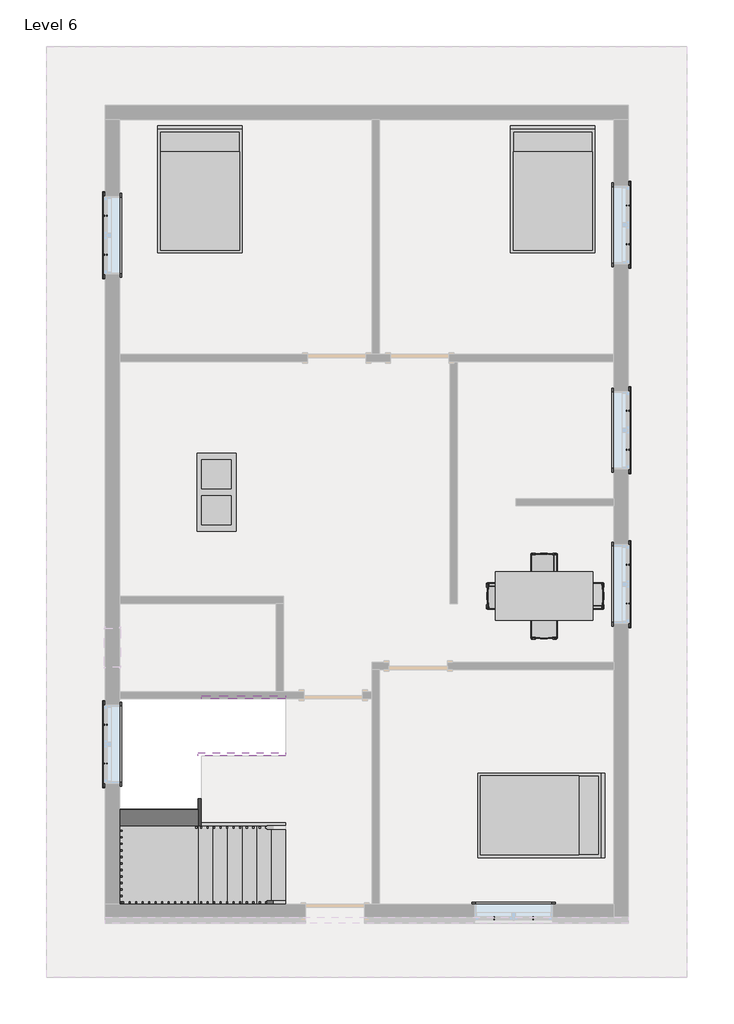
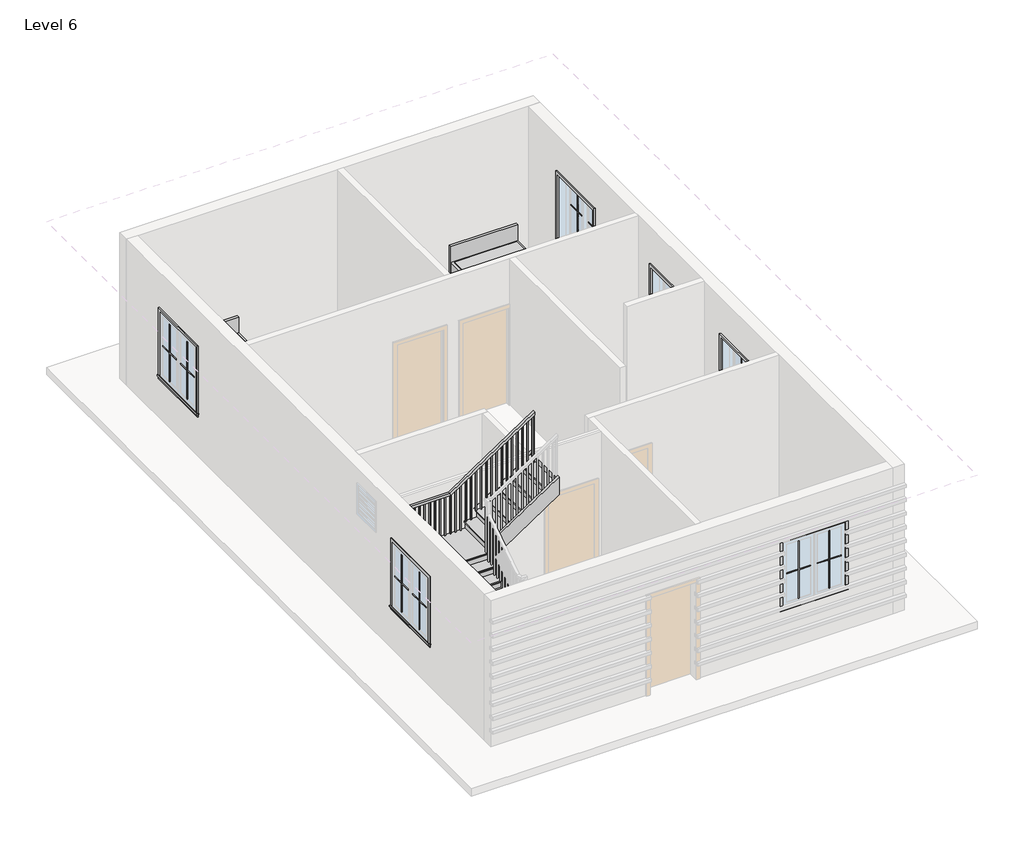
# One storey, part 3 of 3: 25 proxies, 5 members, 4 furniture elements, 1 railing, 1 stair flight.
"""IFC4 building model written with IfcOpenShell, lengths in millimetres."""

from ifc_helpers import new_model, si_unit, frame, origin, place, context, project, spatial, polyline, outline, extrude, faceted_brep, transform, mapped, element, save
from components import muntin_pattern_2x2_muntin_pattern_2x2_ba8901dc, muntin_pattern_2x2_muntin_pattern_2x2_877df4e9, trim_window_exterior_flat_with_sill_fda35bc9, trim_window_interior_flat_picture_frame_a80dbcd9, coffee_table_with_brass_mullions_11320_coffee_table_with_5962bef7, bed_17739_bed_17739_15c61121, dining_table_w_chairs_11374_0cdfc61b, stair_flight_f9fade56

model = new_model("IFC4")

# Units and contexts
model_context = context("Model", 3, world=origin())
ifc_project = project(units=[si_unit("LENGTHUNIT", "METRE", prefix="MILLI")], contexts=[model_context])

# Site, building, storey
site = spatial("IfcSite", under=ifc_project)
building = spatial("IfcBuilding", under=site)
storey = spatial("IfcBuildingStorey", under=building, Name="Level 6", Elevation=15849.6)

# Proxies
placement = place(None, origin())
muntin_pattern_2x2_muntin_pattern_2x2_shape = muntin_pattern_2x2_muntin_pattern_2x2_ba8901dc(model_context)
element("IfcBuildingElementProxy", 1, Name="Muntin Pattern_2x2 : Muntin Pattern_2x2", ObjectType="Muntin Pattern_2x2 : Muntin Pattern_2x2", at=placement, inside=storey, context=model_context, shape_type="MappedRepresentation", body=[
    mapped(muntin_pattern_2x2_muntin_pattern_2x2_shape, transform((-5325.0867403, -4189.9051559, 16833.85), x_axis=(0.0, 1.0, 0.0), y_axis=(-1.0, 0.0, 0.0), z_axis=(0.0, 0.0, 1.0))),
])
element("IfcBuildingElementProxy", 2, Name="Muntin Pattern_2x2 : Muntin Pattern_2x2", ObjectType="Muntin Pattern_2x2 : Muntin Pattern_2x2", at=placement, inside=storey, context=model_context, shape_type="MappedRepresentation", body=[
    mapped(muntin_pattern_2x2_muntin_pattern_2x2_shape, transform((-5325.0867403, 3744.4198441, 16833.85), x_axis=(0.0, 1.0, 0.0), y_axis=(-1.0, 0.0, 0.0), z_axis=(0.0, 0.0, 1.0))),
])
element("IfcBuildingElementProxy", 3, Name="Muntin Pattern_2x2 : Muntin Pattern_2x2", ObjectType="Muntin Pattern_2x2 : Muntin Pattern_2x2", at=placement, inside=storey, context=model_context, shape_type="MappedRepresentation", body=[
    mapped(muntin_pattern_2x2_muntin_pattern_2x2_shape, transform((2821.9632597, 4512.7698441, 16833.85), x_axis=(0.0, -1.0, 0.0), y_axis=(1.0, 0.0, 0.0), z_axis=(0.0, 0.0, 1.0))),
])
element("IfcBuildingElementProxy", 4, Name="Muntin Pattern_2x2 : Muntin Pattern_2x2", ObjectType="Muntin Pattern_2x2 : Muntin Pattern_2x2", at=placement, inside=storey, context=model_context, shape_type="MappedRepresentation", body=[
    mapped(muntin_pattern_2x2_muntin_pattern_2x2_shape, transform((2821.9632597, 1312.3698441, 16833.85), x_axis=(0.0, -1.0, 0.0), y_axis=(1.0, 0.0, 0.0), z_axis=(0.0, 0.0, 1.0))),
])
element("IfcBuildingElementProxy", 5, Name="Muntin Pattern_2x2 : Muntin Pattern_2x2", ObjectType="Muntin Pattern_2x2 : Muntin Pattern_2x2", at=placement, inside=storey, context=model_context, shape_type="MappedRepresentation", body=[
    mapped(muntin_pattern_2x2_muntin_pattern_2x2_shape, transform((2821.9632597, -1087.9301559, 16833.85), x_axis=(0.0, -1.0, 0.0), y_axis=(1.0, 0.0, 0.0), z_axis=(0.0, 0.0, 1.0))),
])
element("IfcBuildingElementProxy", 6, Name="Muntin Pattern_2x2 : Muntin Pattern_2x2", ObjectType="Muntin Pattern_2x2 : Muntin Pattern_2x2", at=placement, inside=storey, context=model_context, shape_type="MappedRepresentation", body=[
    mapped(muntin_pattern_2x2_muntin_pattern_2x2_shape, transform((1344.0007597, -6601.3176559, 16833.85), x_axis=(-1.0, 0.0, 0.0), y_axis=(0.0, -1.0, 0.0), z_axis=(0.0, 0.0, 1.0))),
])
muntin_pattern_2x2_muntin_pattern_2x2_2_shape = muntin_pattern_2x2_muntin_pattern_2x2_877df4e9(model_context)
element("IfcBuildingElementProxy", 7, Name="Muntin Pattern_2x2 : Muntin Pattern_2x2", ObjectType="Muntin Pattern_2x2 : Muntin Pattern_2x2", at=placement, inside=storey, context=model_context, shape_type="MappedRepresentation", body=[
    mapped(muntin_pattern_2x2_muntin_pattern_2x2_2_shape, transform((-5325.0867403, -3583.4801559, 16833.85), x_axis=(0.0, -1.0, 0.0), y_axis=(1.0, 0.0, 0.0), z_axis=(0.0, 0.0, 1.0))),
])
element("IfcBuildingElementProxy", 8, Name="Muntin Pattern_2x2 : Muntin Pattern_2x2", ObjectType="Muntin Pattern_2x2 : Muntin Pattern_2x2", at=placement, inside=storey, context=model_context, shape_type="MappedRepresentation", body=[
    mapped(muntin_pattern_2x2_muntin_pattern_2x2_2_shape, transform((-5325.0867403, 4350.8448441, 16833.85), x_axis=(0.0, -1.0, 0.0), y_axis=(1.0, 0.0, 0.0), z_axis=(0.0, 0.0, 1.0))),
])
element("IfcBuildingElementProxy", 9, Name="Muntin Pattern_2x2 : Muntin Pattern_2x2", ObjectType="Muntin Pattern_2x2 : Muntin Pattern_2x2", at=placement, inside=storey, context=model_context, shape_type="MappedRepresentation", body=[
    mapped(muntin_pattern_2x2_muntin_pattern_2x2_2_shape, transform((2821.9632597, 3906.3448441, 16833.85), x_axis=(0.0, 1.0, 0.0), y_axis=(-1.0, 0.0, 0.0), z_axis=(0.0, 0.0, 1.0))),
])
element("IfcBuildingElementProxy", 10, Name="Muntin Pattern_2x2 : Muntin Pattern_2x2", ObjectType="Muntin Pattern_2x2 : Muntin Pattern_2x2", at=placement, inside=storey, context=model_context, shape_type="MappedRepresentation", body=[
    mapped(muntin_pattern_2x2_muntin_pattern_2x2_2_shape, transform((2821.9632597, 705.9448441, 16833.85), x_axis=(0.0, 1.0, 0.0), y_axis=(-1.0, 0.0, 0.0), z_axis=(0.0, 0.0, 1.0))),
])
element("IfcBuildingElementProxy", 11, Name="Muntin Pattern_2x2 : Muntin Pattern_2x2", ObjectType="Muntin Pattern_2x2 : Muntin Pattern_2x2", at=placement, inside=storey, context=model_context, shape_type="MappedRepresentation", body=[
    mapped(muntin_pattern_2x2_muntin_pattern_2x2_2_shape, transform((2821.9632597, -1694.3551559, 16833.85), x_axis=(0.0, 1.0, 0.0), y_axis=(-1.0, 0.0, 0.0), z_axis=(0.0, 0.0, 1.0))),
])
element("IfcBuildingElementProxy", 12, Name="Muntin Pattern_2x2 : Muntin Pattern_2x2", ObjectType="Muntin Pattern_2x2 : Muntin Pattern_2x2", at=placement, inside=storey, context=model_context, shape_type="MappedRepresentation", body=[
    mapped(muntin_pattern_2x2_muntin_pattern_2x2_2_shape, transform((737.5757597, -6601.3176559, 16833.85), x_axis=(1.0, 0.0, 0.0), y_axis=(0.0, 1.0, 0.0), z_axis=(0.0, 0.0, 1.0))),
])
trim_window_exterior_flat_with_sill_shape = trim_window_exterior_flat_with_sill_fda35bc9(model_context)
element("IfcBuildingElementProxy", 13, Name="Trim-Window-Exterior-Flat : with Sill", ObjectType="Trim-Window-Exterior-Flat : with Sill", at=placement, inside=storey, context=model_context, shape_type="MappedRepresentation", body=[
    mapped(trim_window_exterior_flat_with_sill_shape, transform((-5334.6117403, -3886.6926559, 18110.2), x_axis=(0.0, -1.0, 0.0), y_axis=(0.0, 0.0, 1.0), z_axis=(-1.0, 0.0, 0.0))),
])
element("IfcBuildingElementProxy", 14, Name="Trim-Window-Exterior-Flat : with Sill", ObjectType="Trim-Window-Exterior-Flat : with Sill", at=placement, inside=storey, context=model_context, shape_type="MappedRepresentation", body=[
    mapped(trim_window_exterior_flat_with_sill_shape, transform((-5334.6117403, 4047.6323441, 18110.2), x_axis=(0.0, -1.0, 0.0), y_axis=(0.0, 0.0, 1.0), z_axis=(-1.0, 0.0, 0.0))),
])
element("IfcBuildingElementProxy", 15, Name="Trim-Window-Exterior-Flat : with Sill", ObjectType="Trim-Window-Exterior-Flat : with Sill", at=placement, inside=storey, context=model_context, shape_type="MappedRepresentation", body=[
    mapped(trim_window_exterior_flat_with_sill_shape, transform((2831.4882597, 4209.5573441, 18110.2), x_axis=(0.0, 1.0, 0.0), y_axis=(0.0, 0.0, 1.0), z_axis=(1.0, 0.0, 0.0))),
])
element("IfcBuildingElementProxy", 16, Name="Trim-Window-Exterior-Flat : with Sill", ObjectType="Trim-Window-Exterior-Flat : with Sill", at=placement, inside=storey, context=model_context, shape_type="MappedRepresentation", body=[
    mapped(trim_window_exterior_flat_with_sill_shape, transform((2831.4882597, 1009.1573441, 18110.2), x_axis=(0.0, 1.0, 0.0), y_axis=(0.0, 0.0, 1.0), z_axis=(1.0, 0.0, 0.0))),
])
element("IfcBuildingElementProxy", 17, Name="Trim-Window-Exterior-Flat : with Sill", ObjectType="Trim-Window-Exterior-Flat : with Sill", at=placement, inside=storey, context=model_context, shape_type="MappedRepresentation", body=[
    mapped(trim_window_exterior_flat_with_sill_shape, transform((2831.4882597, -1391.1426559, 18110.2), x_axis=(0.0, 1.0, 0.0), y_axis=(0.0, 0.0, 1.0), z_axis=(1.0, 0.0, 0.0))),
])
element("IfcBuildingElementProxy", 18, Name="Trim-Window-Exterior-Flat : with Sill", ObjectType="Trim-Window-Exterior-Flat : with Sill", at=placement, inside=storey, context=model_context, shape_type="MappedRepresentation", body=[
    mapped(trim_window_exterior_flat_with_sill_shape, transform((1040.7882597, -6610.8426559, 18110.2), x_axis=(1.0, 0.0, 0.0), y_axis=(0.0, 0.0, 1.0), z_axis=(0.0, -1.0, 0.0))),
])
trim_window_interior_flat_picture_frame_shape = trim_window_interior_flat_picture_frame_a80dbcd9(model_context)
element("IfcBuildingElementProxy", 19, Name="Trim-Window-Interior-Flat : Picture Frame", ObjectType="Trim-Window-Interior-Flat : Picture Frame", at=placement, inside=storey, context=model_context, shape_type="MappedRepresentation", body=[
    mapped(trim_window_interior_flat_picture_frame_shape, transform((-5106.0117403, -3886.6926559, 18110.2), x_axis=(0.0, 1.0, 0.0), y_axis=(0.0, 0.0, 1.0), z_axis=(1.0, 0.0, 0.0))),
])
element("IfcBuildingElementProxy", 20, Name="Trim-Window-Interior-Flat : Picture Frame", ObjectType="Trim-Window-Interior-Flat : Picture Frame", at=placement, inside=storey, context=model_context, shape_type="MappedRepresentation", body=[
    mapped(trim_window_interior_flat_picture_frame_shape, transform((-5106.0117403, 4047.6323441, 18110.2), x_axis=(0.0, 1.0, 0.0), y_axis=(0.0, 0.0, 1.0), z_axis=(1.0, 0.0, 0.0))),
])
element("IfcBuildingElementProxy", 21, Name="Trim-Window-Interior-Flat : Picture Frame", ObjectType="Trim-Window-Interior-Flat : Picture Frame", at=placement, inside=storey, context=model_context, shape_type="MappedRepresentation", body=[
    mapped(trim_window_interior_flat_picture_frame_shape, transform((2602.8882597, 4209.5573441, 18110.2), x_axis=(0.0, -1.0, 0.0), y_axis=(0.0, 0.0, 1.0), z_axis=(-1.0, 0.0, 0.0))),
])
element("IfcBuildingElementProxy", 22, Name="Trim-Window-Interior-Flat : Picture Frame", ObjectType="Trim-Window-Interior-Flat : Picture Frame", at=placement, inside=storey, context=model_context, shape_type="MappedRepresentation", body=[
    mapped(trim_window_interior_flat_picture_frame_shape, transform((2602.8882597, 1009.1573441, 18110.2), x_axis=(0.0, -1.0, 0.0), y_axis=(0.0, 0.0, 1.0), z_axis=(-1.0, 0.0, 0.0))),
])
element("IfcBuildingElementProxy", 23, Name="Trim-Window-Interior-Flat : Picture Frame", ObjectType="Trim-Window-Interior-Flat : Picture Frame", at=placement, inside=storey, context=model_context, shape_type="MappedRepresentation", body=[
    mapped(trim_window_interior_flat_picture_frame_shape, transform((2602.8882597, -1391.1426559, 18110.2), x_axis=(0.0, -1.0, 0.0), y_axis=(0.0, 0.0, 1.0), z_axis=(-1.0, 0.0, 0.0))),
])
element("IfcBuildingElementProxy", 24, Name="Trim-Window-Interior-Flat : Picture Frame", ObjectType="Trim-Window-Interior-Flat : Picture Frame", at=placement, inside=storey, context=model_context, shape_type="MappedRepresentation", body=[
    mapped(trim_window_interior_flat_picture_frame_shape, transform((1040.7882597, -6382.2426559, 18110.2), x_axis=(-1.0, 0.0, 0.0), y_axis=(0.0, 0.0, 1.0), z_axis=(0.0, 1.0, 0.0))),
])
coffee_table_with_brass_mullions_11320_coffee_table_with_shape = coffee_table_with_brass_mullions_11320_coffee_table_with_5962bef7(model_context)
element("IfcBuildingElementProxy", 25, Name="coffee_table_with_brass_mullions_11320 : coffee_table_with_brass_mullions_11320", ObjectType="coffee_table_with_brass_mullions_11320 : coffee_table_with_brass_mullions_11320", at=placement, inside=storey, context=model_context, shape_type="MappedRepresentation", body=[
    mapped(coffee_table_with_brass_mullions_11320_coffee_table_with_shape, transform((-3162.9117403, 678.9573441, 15849.6), x_axis=(0.0, 1.0, 0.0), y_axis=(-1.0, 0.0, 0.0), z_axis=(0.0, 0.0, 1.0))),
])

# Furniture
bed_17739_bed_17739_shape = bed_17739_bed_17739_15c61121(model_context)
element("IfcFurniture", 26, ObjectType="Bed_17739 : Bed_17739", at=placement, inside=storey, context=model_context, shape_type="MappedRepresentation", body=[
    mapped(bed_17739_bed_17739_shape, transform((-3855.0617403, 4742.9573441, 15849.6), x_axis=(1.0, 0.0, 0.0), y_axis=(0.0, 1.0, 0.0), z_axis=(0.0, 0.0, 1.0))),
])
element("IfcFurniture", 27, ObjectType="Bed_17739 : Bed_17739", at=placement, inside=storey, context=model_context, shape_type="MappedRepresentation", body=[
    mapped(bed_17739_bed_17739_shape, transform((1650.3882597, 4742.9573441, 15849.6), x_axis=(1.0, 0.0, 0.0), y_axis=(0.0, 1.0, 0.0), z_axis=(0.0, 0.0, 1.0))),
])
element("IfcFurniture", 28, ObjectType="Bed_17739 : Bed_17739", at=placement, inside=storey, context=model_context, shape_type="MappedRepresentation", body=[
    mapped(bed_17739_bed_17739_shape, transform((1447.1882597, -4997.9426559, 15849.6), x_axis=(0.0, -1.0, 0.0), y_axis=(1.0, 0.0, 0.0), z_axis=(0.0, 0.0, 1.0))),
])
dining_table_w_chairs_11374_shape = dining_table_w_chairs_11374_0cdfc61b(model_context)
element("IfcFurniture", 29, ObjectType="Dining_Table_w_Chairs_11374", at=placement, inside=storey, context=model_context, shape_type="MappedRepresentation", body=[
    mapped(dining_table_w_chairs_11374_shape, transform((1497.0410232, -1671.6886654, 15849.6), x_axis=(1.0, 0.0, 0.0), y_axis=(0.0, 1.0, 0.0), z_axis=(0.0, 0.0, 1.0))),
])

# Members
element("IfcMember", 30, ObjectType="Stringer - 2\" Width", at=placement, inside=storey, context=model_context, shape_type="SweptSolid", body=[
    extrude(outline(polyline([(15849.6, -2515.2117403), (16067.6398409, -2515.2117403), (16321.6398409, -2896.2117403), (16321.6398409, -3445.6977546), (15849.6, -2737.6379933), (15849.6, -2515.2117403)])), frame((0.0, -6433.0426559, 0.0), z_axis=(0.0, 1.0, 0.0), x_axis=(0.0, 0.0, 1.0)), (0.0, 0.0, 1.0), 50.8),
])
element("IfcMember", 31, ObjectType="Stringer - 2\" Width", at=placement, inside=storey, context=model_context, shape_type="SweptSolid", body=[
    extrude(outline(polyline([(18088.9158313, -3277.2117403), (18596.9158313, -2515.2117403), (18963.2398409, -2515.2117403), (18088.9158313, -3826.6977546), (18088.9158313, -3277.2117403)])), frame((0.0, -3181.8426559, 0.0), z_axis=(0.0, 1.0, 0.0), x_axis=(0.0, 0.0, 1.0)), (0.0, 0.0, 1.0), 50.8),
])
element("IfcMember", 32, ObjectType="Stringer - 2\" Width", at=placement, inside=storey, context=model_context, shape_type="SweptSolid", body=[
    extrude(outline(polyline([(15849.6, -2515.2117403), (16067.6398409, -2515.2117403), (16948.1731743, -3836.0117403), (16581.8491647, -3836.0117403), (15849.6, -2737.6379933), (15849.6, -2515.2117403)])), frame((0.0, -5163.0426559, 0.0), z_axis=(0.0, 1.0, 0.0), x_axis=(0.0, 0.0, 1.0)), (0.0, 0.0, 1.0), 50.8),
])
element("IfcMember", 33, ObjectType="Stringer - 2\" Width", at=placement, inside=storey, context=model_context, shape_type="SweptSolid", body=[
    extrude(outline(polyline([(-5163.0426559, 16768.1158313), (-5163.0426559, 17134.4398409), (-4070.8426559, 17862.5731743), (-4070.8426559, 17496.2491647), (-5163.0426559, 16768.1158313)])), frame((-3886.8117403, 0.0, 0.0), z_axis=(1.0, 0.0, 0.0), x_axis=(0.0, 1.0, 0.0)), (0.0, 0.0, 1.0), 50.8),
])
element("IfcMember", 34, ObjectType="Stringer - 2\" Width", at=placement, inside=storey, context=model_context, shape_type="SweptSolid", body=[
    extrude(outline(polyline([(18048.8398409, -3886.8117403), (17682.5158313, -3886.8117403), (18596.9158313, -2515.2117403), (18963.2398409, -2515.2117403), (18048.8398409, -3886.8117403)])), frame((0.0, -4070.8426559, 0.0), z_axis=(0.0, 1.0, 0.0), x_axis=(0.0, 0.0, 1.0)), (0.0, 0.0, 1.0), 50.8),
])

# Railing
element("IfcRailing", 35, ObjectType="Handrail - Rectangular", at=placement, inside=storey, context=model_context, shape_type="SolidModel", body=[
    faceted_brep([(-2515.2117403, -6382.2426559, 16916.4), (-2515.2117403, -6382.2426559, 16855.3459984), (-2515.2117403, -6331.4426559, 16855.3459984), (-2515.2117403, -6331.4426559, 16916.4), (-4001.1117403, -6382.2426559, 17907.0), (-4016.4927427, -6382.2426559, 17856.2), (-4016.4927427, -6331.4426559, 17856.2), (-4001.1117403, -6331.4426559, 17907.0), (-5106.0117403, -6382.2426559, 17907.0), (-5106.0117403, -6382.2426559, 17856.2), (-5055.2117403, -6331.4426559, 17856.2), (-5055.2117403, -6331.4426559, 17907.0), (-5106.0117403, -5277.3426559, 17907.0), (-5106.0117403, -5261.9616535, 17856.2), (-5055.2117403, -5261.9616535, 17856.2), (-5055.2117403, -5277.3426559, 17907.0), (-5106.0117403, -4096.2426559, 18694.4), (-5106.0117403, -4080.8616535, 18643.6), (-5055.2117403, -4080.8616535, 18643.6), (-5055.2117403, -4096.2426559, 18694.4), (-5106.0117403, -3181.8426559, 18694.4), (-5106.0117403, -3181.8426559, 18643.6), (-5055.2117403, -3232.6426559, 18643.6), (-5055.2117403, -3232.6426559, 18694.4), (-4191.6117403, -3181.8426559, 18694.4), (-4176.2307379, -3181.8426559, 18643.6), (-4176.2307379, -3232.6426559, 18643.6), (-4191.6117403, -3232.6426559, 18694.4), (-2515.2117403, -3181.8426559, 19812.0), (-2515.2117403, -3232.6426559, 19812.0), (-2515.2117403, -3232.6426559, 19750.9459984), (-2515.2117403, -3181.8426559, 19750.9459984)], [[[0, 1, 2, 3]], [[1, 0, 4, 5]], [[2, 1, 5, 6]], [[3, 2, 6, 7]], [[0, 3, 7, 4]], [[5, 4, 8, 9]], [[6, 5, 9, 10]], [[7, 6, 10, 11]], [[4, 7, 11, 8]], [[9, 8, 12, 13]], [[10, 9, 13, 14]], [[11, 10, 14, 15]], [[8, 11, 15, 12]], [[13, 12, 16, 17]], [[14, 13, 17, 18]], [[15, 14, 18, 19]], [[12, 15, 19, 16]], [[17, 16, 20, 21]], [[18, 17, 21, 22]], [[19, 18, 22, 23]], [[16, 19, 23, 20]], [[21, 20, 24, 25]], [[22, 21, 25, 26]], [[23, 22, 26, 27]], [[20, 23, 27, 24]], [[28, 29, 30, 31]], [[25, 24, 28, 31]], [[26, 25, 31, 30]], [[27, 26, 30, 29]], [[24, 27, 29, 28]]]),
    extrude(outline(polyline([(19727.6626651, -2550.1367403), (18745.2, -2550.1367403), (18745.2, -2531.0867403), (19740.3626651, -2531.0867403), (19727.6626651, -2550.1367403)])), frame((0.0, -3216.7676559, 0.0), z_axis=(0.0, 1.0, 0.0), x_axis=(0.0, 0.0, 1.0)), (0.0, 0.0, 1.0), 19.05),
    extrude(outline(polyline([(19659.9293317, -2651.7367403), (18745.2, -2651.7367403), (18745.2, -2632.6867403), (19672.6293317, -2632.6867403), (19659.9293317, -2651.7367403)])), frame((0.0, -3216.7676559, 0.0), z_axis=(0.0, 1.0, 0.0), x_axis=(0.0, 0.0, 1.0)), (0.0, 0.0, 1.0), 19.05),
    extrude(outline(polyline([(19592.1959984, -2753.3367403), (18745.2, -2753.3367403), (18745.2, -2734.2867403), (19604.8959984, -2734.2867403), (19592.1959984, -2753.3367403)])), frame((0.0, -3216.7676559, 0.0), z_axis=(0.0, 1.0, 0.0), x_axis=(0.0, 0.0, 1.0)), (0.0, 0.0, 1.0), 19.05),
    extrude(outline(polyline([(19524.4626651, -2854.9367403), (18592.8, -2854.9367403), (18592.8, -2835.8867403), (19537.1626651, -2835.8867403), (19524.4626651, -2854.9367403)])), frame((0.0, -3216.7676559, 0.0), z_axis=(0.0, 1.0, 0.0), x_axis=(0.0, 0.0, 1.0)), (0.0, 0.0, 1.0), 19.05),
    extrude(outline(polyline([(19456.7293317, -2956.5367403), (18592.8, -2956.5367403), (18592.8, -2937.4867403), (19469.4293317, -2937.4867403), (19456.7293317, -2956.5367403)])), frame((0.0, -3216.7676559, 0.0), z_axis=(0.0, 1.0, 0.0), x_axis=(0.0, 0.0, 1.0)), (0.0, 0.0, 1.0), 19.05),
    extrude(outline(polyline([(19388.9959984, -3058.1367403), (18440.4, -3058.1367403), (18440.4, -3039.0867403), (19401.6959984, -3039.0867403), (19388.9959984, -3058.1367403)])), frame((0.0, -3216.7676559, 0.0), z_axis=(0.0, 1.0, 0.0), x_axis=(0.0, 0.0, 1.0)), (0.0, 0.0, 1.0), 19.05),
    extrude(outline(polyline([(19321.2626651, -3159.7367403), (18440.4, -3159.7367403), (18440.4, -3140.6867403), (19333.9626651, -3140.6867403), (19321.2626651, -3159.7367403)])), frame((0.0, -3216.7676559, 0.0), z_axis=(0.0, 1.0, 0.0), x_axis=(0.0, 0.0, 1.0)), (0.0, 0.0, 1.0), 19.05),
    extrude(outline(polyline([(19253.5293317, -3261.3367403), (18288.0, -3261.3367403), (18288.0, -3242.2867403), (19266.2293317, -3242.2867403), (19253.5293317, -3261.3367403)])), frame((0.0, -3216.7676559, 0.0), z_axis=(0.0, 1.0, 0.0), x_axis=(0.0, 0.0, 1.0)), (0.0, 0.0, 1.0), 19.05),
    extrude(outline(polyline([(19185.7959984, -3362.9367403), (18288.0, -3362.9367403), (18288.0, -3343.8867403), (19198.4959984, -3343.8867403), (19185.7959984, -3362.9367403)])), frame((0.0, -3216.7676559, 0.0), z_axis=(0.0, 1.0, 0.0), x_axis=(0.0, 0.0, 1.0)), (0.0, 0.0, 1.0), 19.05),
    extrude(outline(polyline([(19118.0626651, -3464.5367403), (18135.6, -3464.5367403), (18135.6, -3445.4867403), (19130.7626651, -3445.4867403), (19118.0626651, -3464.5367403)])), frame((0.0, -3216.7676559, 0.0), z_axis=(0.0, 1.0, 0.0), x_axis=(0.0, 0.0, 1.0)), (0.0, 0.0, 1.0), 19.05),
    extrude(outline(polyline([(19050.3293317, -3566.1367403), (18135.6, -3566.1367403), (18135.6, -3547.0867403), (19063.0293317, -3547.0867403), (19050.3293317, -3566.1367403)])), frame((0.0, -3216.7676559, 0.0), z_axis=(0.0, 1.0, 0.0), x_axis=(0.0, 0.0, 1.0)), (0.0, 0.0, 1.0), 19.05),
    extrude(outline(polyline([(18982.5959984, -3667.7367403), (18135.6, -3667.7367403), (18135.6, -3648.6867403), (18995.2959984, -3648.6867403), (18982.5959984, -3667.7367403)])), frame((0.0, -3216.7676559, 0.0), z_axis=(0.0, 1.0, 0.0), x_axis=(0.0, 0.0, 1.0)), (0.0, 0.0, 1.0), 19.05),
    extrude(outline(polyline([(18914.8626651, -3769.3367403), (17983.2, -3769.3367403), (17983.2, -3750.2867403), (18927.5626651, -3750.2867403), (18914.8626651, -3769.3367403)])), frame((0.0, -3216.7676559, 0.0), z_axis=(0.0, 1.0, 0.0), x_axis=(0.0, 0.0, 1.0)), (0.0, 0.0, 1.0), 19.05),
    extrude(outline(polyline([(18847.1293317, -3870.9367403), (17983.2, -3870.9367403), (17983.2, -3851.8867403), (18859.8293317, -3851.8867403), (18847.1293317, -3870.9367403)])), frame((0.0, -3216.7676559, 0.0), z_axis=(0.0, 1.0, 0.0), x_axis=(0.0, 0.0, 1.0)), (0.0, 0.0, 1.0), 19.05),
    extrude(outline(polyline([(18779.3959984, -3972.5367403), (17830.8, -3972.5367403), (17830.8, -3953.4867403), (18792.0959984, -3953.4867403), (18779.3959984, -3972.5367403)])), frame((0.0, -3216.7676559, 0.0), z_axis=(0.0, 1.0, 0.0), x_axis=(0.0, 0.0, 1.0)), (0.0, 0.0, 1.0), 19.05),
    extrude(outline(polyline([(18711.6626651, -4074.1367403), (17830.8, -4074.1367403), (17830.8, -4055.0867403), (18724.3626651, -4055.0867403), (18711.6626651, -4074.1367403)])), frame((0.0, -3216.7676559, 0.0), z_axis=(0.0, 1.0, 0.0), x_axis=(0.0, 0.0, 1.0)), (0.0, 0.0, 1.0), 19.05),
    extrude(outline(polyline([(18643.9293317, -4175.7367403), (17830.8, -4175.7367403), (17830.8, -4156.6867403), (18656.6293317, -4156.6867403), (18643.9293317, -4175.7367403)])), frame((0.0, -3216.7676559, 0.0), z_axis=(0.0, 1.0, 0.0), x_axis=(0.0, 0.0, 1.0)), (0.0, 0.0, 1.0), 19.05),
    extrude(outline(polyline([(-4277.3367403, -3197.7176559), (-4258.2867403, -3197.7176559), (-4258.2867403, -3216.7676559), (-4277.3367403, -3216.7676559), (-4277.3367403, -3197.7176559)])), frame((0.0, 0.0, 17830.8), z_axis=(0.0, 0.0, 1.0), x_axis=(1.0, 0.0, 0.0)), (0.0, 0.0, 1.0), 812.8),
    extrude(outline(polyline([(-4378.9367403, -3197.7176559), (-4359.8867403, -3197.7176559), (-4359.8867403, -3216.7676559), (-4378.9367403, -3216.7676559), (-4378.9367403, -3197.7176559)])), frame((0.0, 0.0, 17830.8), z_axis=(0.0, 0.0, 1.0), x_axis=(1.0, 0.0, 0.0)), (0.0, 0.0, 1.0), 812.8),
    extrude(outline(polyline([(-4480.5367403, -3197.7176559), (-4461.4867403, -3197.7176559), (-4461.4867403, -3216.7676559), (-4480.5367403, -3216.7676559), (-4480.5367403, -3197.7176559)])), frame((0.0, 0.0, 17830.8), z_axis=(0.0, 0.0, 1.0), x_axis=(1.0, 0.0, 0.0)), (0.0, 0.0, 1.0), 812.8),
    extrude(outline(polyline([(-4582.1367403, -3197.7176559), (-4563.0867403, -3197.7176559), (-4563.0867403, -3216.7676559), (-4582.1367403, -3216.7676559), (-4582.1367403, -3197.7176559)])), frame((0.0, 0.0, 17830.8), z_axis=(0.0, 0.0, 1.0), x_axis=(1.0, 0.0, 0.0)), (0.0, 0.0, 1.0), 812.8),
    extrude(outline(polyline([(-4683.7367403, -3197.7176559), (-4664.6867403, -3197.7176559), (-4664.6867403, -3216.7676559), (-4683.7367403, -3216.7676559), (-4683.7367403, -3197.7176559)])), frame((0.0, 0.0, 17830.8), z_axis=(0.0, 0.0, 1.0), x_axis=(1.0, 0.0, 0.0)), (0.0, 0.0, 1.0), 812.8),
    extrude(outline(polyline([(-4785.3367403, -3197.7176559), (-4766.2867403, -3197.7176559), (-4766.2867403, -3216.7676559), (-4785.3367403, -3216.7676559), (-4785.3367403, -3197.7176559)])), frame((0.0, 0.0, 17830.8), z_axis=(0.0, 0.0, 1.0), x_axis=(1.0, 0.0, 0.0)), (0.0, 0.0, 1.0), 812.8),
    extrude(outline(polyline([(-4886.9367403, -3197.7176559), (-4867.8867403, -3197.7176559), (-4867.8867403, -3216.7676559), (-4886.9367403, -3216.7676559), (-4886.9367403, -3197.7176559)])), frame((0.0, 0.0, 17830.8), z_axis=(0.0, 0.0, 1.0), x_axis=(1.0, 0.0, 0.0)), (0.0, 0.0, 1.0), 812.8),
    extrude(outline(polyline([(-4988.5367403, -3197.7176559), (-4969.4867403, -3197.7176559), (-4969.4867403, -3216.7676559), (-4988.5367403, -3216.7676559), (-4988.5367403, -3197.7176559)])), frame((0.0, 0.0, 17830.8), z_axis=(0.0, 0.0, 1.0), x_axis=(1.0, 0.0, 0.0)), (0.0, 0.0, 1.0), 812.8),
    extrude(outline(polyline([(-5090.1367403, -3318.3676559), (-5090.1367403, -3299.3176559), (-5071.0867403, -3299.3176559), (-5071.0867403, -3318.3676559), (-5090.1367403, -3318.3676559)])), frame((0.0, 0.0, 17830.8), z_axis=(0.0, 0.0, 1.0), x_axis=(1.0, 0.0, 0.0)), (0.0, 0.0, 1.0), 812.8),
    extrude(outline(polyline([(-5090.1367403, -3419.9676559), (-5090.1367403, -3400.9176559), (-5071.0867403, -3400.9176559), (-5071.0867403, -3419.9676559), (-5090.1367403, -3419.9676559)])), frame((0.0, 0.0, 17830.8), z_axis=(0.0, 0.0, 1.0), x_axis=(1.0, 0.0, 0.0)), (0.0, 0.0, 1.0), 812.8),
    extrude(outline(polyline([(-5090.1367403, -3521.5676559), (-5090.1367403, -3502.5176559), (-5071.0867403, -3502.5176559), (-5071.0867403, -3521.5676559), (-5090.1367403, -3521.5676559)])), frame((0.0, 0.0, 17830.8), z_axis=(0.0, 0.0, 1.0), x_axis=(1.0, 0.0, 0.0)), (0.0, 0.0, 1.0), 812.8),
    extrude(outline(polyline([(-5090.1367403, -3623.1676559), (-5090.1367403, -3604.1176559), (-5071.0867403, -3604.1176559), (-5071.0867403, -3623.1676559), (-5090.1367403, -3623.1676559)])), frame((0.0, 0.0, 17830.8), z_axis=(0.0, 0.0, 1.0), x_axis=(1.0, 0.0, 0.0)), (0.0, 0.0, 1.0), 812.8),
    extrude(outline(polyline([(-5090.1367403, -3724.7676559), (-5090.1367403, -3705.7176559), (-5071.0867403, -3705.7176559), (-5071.0867403, -3724.7676559), (-5090.1367403, -3724.7676559)])), frame((0.0, 0.0, 17830.8), z_axis=(0.0, 0.0, 1.0), x_axis=(1.0, 0.0, 0.0)), (0.0, 0.0, 1.0), 812.8),
    extrude(outline(polyline([(-5090.1367403, -3826.3676559), (-5090.1367403, -3807.3176559), (-5071.0867403, -3807.3176559), (-5071.0867403, -3826.3676559), (-5090.1367403, -3826.3676559)])), frame((0.0, 0.0, 17830.8), z_axis=(0.0, 0.0, 1.0), x_axis=(1.0, 0.0, 0.0)), (0.0, 0.0, 1.0), 812.8),
    extrude(outline(polyline([(-5090.1367403, -3927.9676559), (-5090.1367403, -3908.9176559), (-5071.0867403, -3908.9176559), (-5071.0867403, -3927.9676559), (-5090.1367403, -3927.9676559)])), frame((0.0, 0.0, 17830.8), z_axis=(0.0, 0.0, 1.0), x_axis=(1.0, 0.0, 0.0)), (0.0, 0.0, 1.0), 812.8),
    extrude(outline(polyline([(-5090.1367403, -4029.5676559), (-5090.1367403, -4010.5176559), (-5071.0867403, -4010.5176559), (-5071.0867403, -4029.5676559), (-5090.1367403, -4029.5676559)])), frame((0.0, 0.0, 17830.8), z_axis=(0.0, 0.0, 1.0), x_axis=(1.0, 0.0, 0.0)), (0.0, 0.0, 1.0), 812.8),
    extrude(outline(polyline([(-4112.1176559, 18622.7626651), (-4112.1176559, 17678.4), (-4131.1676559, 17678.4), (-4131.1676559, 18610.0626651), (-4112.1176559, 18622.7626651)])), frame((-5090.1367403, 0.0, 0.0), z_axis=(1.0, 0.0, 0.0), x_axis=(0.0, 1.0, 0.0)), (0.0, 0.0, 1.0), 19.05),
    extrude(outline(polyline([(-4213.7176559, 18555.0293317), (-4213.7176559, 17678.4), (-4232.7676559, 17678.4), (-4232.7676559, 18542.3293317), (-4213.7176559, 18555.0293317)])), frame((-5090.1367403, 0.0, 0.0), z_axis=(1.0, 0.0, 0.0), x_axis=(0.0, 1.0, 0.0)), (0.0, 0.0, 1.0), 19.05),
    extrude(outline(polyline([(-4315.3176559, 18487.2959984), (-4315.3176559, 17526.0), (-4334.3676559, 17526.0), (-4334.3676559, 18474.5959984), (-4315.3176559, 18487.2959984)])), frame((-5090.1367403, 0.0, 0.0), z_axis=(1.0, 0.0, 0.0), x_axis=(0.0, 1.0, 0.0)), (0.0, 0.0, 1.0), 19.05),
    extrude(outline(polyline([(-4416.9176559, 18419.5626651), (-4416.9176559, 17526.0), (-4435.9676559, 17526.0), (-4435.9676559, 18406.8626651), (-4416.9176559, 18419.5626651)])), frame((-5090.1367403, 0.0, 0.0), z_axis=(1.0, 0.0, 0.0), x_axis=(0.0, 1.0, 0.0)), (0.0, 0.0, 1.0), 19.05),
    extrude(outline(polyline([(-4518.5176559, 18351.8293317), (-4518.5176559, 17373.6), (-4537.5676559, 17373.6), (-4537.5676559, 18339.1293317), (-4518.5176559, 18351.8293317)])), frame((-5090.1367403, 0.0, 0.0), z_axis=(1.0, 0.0, 0.0), x_axis=(0.0, 1.0, 0.0)), (0.0, 0.0, 1.0), 19.05),
    extrude(outline(polyline([(-4620.1176559, 18284.0959984), (-4620.1176559, 17373.6), (-4639.1676559, 17373.6), (-4639.1676559, 18271.3959984), (-4620.1176559, 18284.0959984)])), frame((-5090.1367403, 0.0, 0.0), z_axis=(1.0, 0.0, 0.0), x_axis=(0.0, 1.0, 0.0)), (0.0, 0.0, 1.0), 19.05),
    extrude(outline(polyline([(-4721.7176559, 18216.3626651), (-4721.7176559, 17221.2), (-4740.7676559, 17221.2), (-4740.7676559, 18203.6626651), (-4721.7176559, 18216.3626651)])), frame((-5090.1367403, 0.0, 0.0), z_axis=(1.0, 0.0, 0.0), x_axis=(0.0, 1.0, 0.0)), (0.0, 0.0, 1.0), 19.05),
    extrude(outline(polyline([(-4823.3176559, 18148.6293317), (-4823.3176559, 17221.2), (-4842.3676559, 17221.2), (-4842.3676559, 18135.9293317), (-4823.3176559, 18148.6293317)])), frame((-5090.1367403, 0.0, 0.0), z_axis=(1.0, 0.0, 0.0), x_axis=(0.0, 1.0, 0.0)), (0.0, 0.0, 1.0), 19.05),
    extrude(outline(polyline([(-4924.9176559, 18080.8959984), (-4924.9176559, 17221.2), (-4943.9676559, 17221.2), (-4943.9676559, 18068.1959984), (-4924.9176559, 18080.8959984)])), frame((-5090.1367403, 0.0, 0.0), z_axis=(1.0, 0.0, 0.0), x_axis=(0.0, 1.0, 0.0)), (0.0, 0.0, 1.0), 19.05),
    extrude(outline(polyline([(-5026.5176559, 18013.1626651), (-5026.5176559, 17068.8), (-5045.5676559, 17068.8), (-5045.5676559, 18000.4626651), (-5026.5176559, 18013.1626651)])), frame((-5090.1367403, 0.0, 0.0), z_axis=(1.0, 0.0, 0.0), x_axis=(0.0, 1.0, 0.0)), (0.0, 0.0, 1.0), 19.05),
    extrude(outline(polyline([(-5128.1176559, 17945.4293317), (-5128.1176559, 17068.8), (-5147.1676559, 17068.8), (-5147.1676559, 17932.7293317), (-5128.1176559, 17945.4293317)])), frame((-5090.1367403, 0.0, 0.0), z_axis=(1.0, 0.0, 0.0), x_axis=(0.0, 1.0, 0.0)), (0.0, 0.0, 1.0), 19.05),
    extrude(outline(polyline([(-5229.7176559, 17877.6959984), (-5229.7176559, 16916.4), (-5248.7676559, 16916.4), (-5248.7676559, 17864.9959984), (-5229.7176559, 17877.6959984)])), frame((-5090.1367403, 0.0, 0.0), z_axis=(1.0, 0.0, 0.0), x_axis=(0.0, 1.0, 0.0)), (0.0, 0.0, 1.0), 19.05),
    extrude(outline(polyline([(-5090.1367403, -5350.3676559), (-5090.1367403, -5331.3176559), (-5071.0867403, -5331.3176559), (-5071.0867403, -5350.3676559), (-5090.1367403, -5350.3676559)])), frame((0.0, 0.0, 16916.4), z_axis=(0.0, 0.0, 1.0), x_axis=(1.0, 0.0, 0.0)), (0.0, 0.0, 1.0), 939.8),
    extrude(outline(polyline([(-5090.1367403, -5451.9676559), (-5090.1367403, -5432.9176559), (-5071.0867403, -5432.9176559), (-5071.0867403, -5451.9676559), (-5090.1367403, -5451.9676559)])), frame((0.0, 0.0, 16916.4), z_axis=(0.0, 0.0, 1.0), x_axis=(1.0, 0.0, 0.0)), (0.0, 0.0, 1.0), 939.8),
    extrude(outline(polyline([(-5090.1367403, -5553.5676559), (-5090.1367403, -5534.5176559), (-5071.0867403, -5534.5176559), (-5071.0867403, -5553.5676559), (-5090.1367403, -5553.5676559)])), frame((0.0, 0.0, 16916.4), z_axis=(0.0, 0.0, 1.0), x_axis=(1.0, 0.0, 0.0)), (0.0, 0.0, 1.0), 939.8),
    extrude(outline(polyline([(-5090.1367403, -5655.1676559), (-5090.1367403, -5636.1176559), (-5071.0867403, -5636.1176559), (-5071.0867403, -5655.1676559), (-5090.1367403, -5655.1676559)])), frame((0.0, 0.0, 16916.4), z_axis=(0.0, 0.0, 1.0), x_axis=(1.0, 0.0, 0.0)), (0.0, 0.0, 1.0), 939.8),
    extrude(outline(polyline([(-5090.1367403, -5756.7676559), (-5090.1367403, -5737.7176559), (-5071.0867403, -5737.7176559), (-5071.0867403, -5756.7676559), (-5090.1367403, -5756.7676559)])), frame((0.0, 0.0, 16916.4), z_axis=(0.0, 0.0, 1.0), x_axis=(1.0, 0.0, 0.0)), (0.0, 0.0, 1.0), 939.8),
    extrude(outline(polyline([(-5090.1367403, -5858.3676559), (-5090.1367403, -5839.3176559), (-5071.0867403, -5839.3176559), (-5071.0867403, -5858.3676559), (-5090.1367403, -5858.3676559)])), frame((0.0, 0.0, 16916.4), z_axis=(0.0, 0.0, 1.0), x_axis=(1.0, 0.0, 0.0)), (0.0, 0.0, 1.0), 939.8),
    extrude(outline(polyline([(-5090.1367403, -5959.9676559), (-5090.1367403, -5940.9176559), (-5071.0867403, -5940.9176559), (-5071.0867403, -5959.9676559), (-5090.1367403, -5959.9676559)])), frame((0.0, 0.0, 16916.4), z_axis=(0.0, 0.0, 1.0), x_axis=(1.0, 0.0, 0.0)), (0.0, 0.0, 1.0), 939.8),
    extrude(outline(polyline([(-5090.1367403, -6061.5676559), (-5090.1367403, -6042.5176559), (-5071.0867403, -6042.5176559), (-5071.0867403, -6061.5676559), (-5090.1367403, -6061.5676559)])), frame((0.0, 0.0, 16916.4), z_axis=(0.0, 0.0, 1.0), x_axis=(1.0, 0.0, 0.0)), (0.0, 0.0, 1.0), 939.8),
    extrude(outline(polyline([(-5090.1367403, -6163.1676559), (-5090.1367403, -6144.1176559), (-5071.0867403, -6144.1176559), (-5071.0867403, -6163.1676559), (-5090.1367403, -6163.1676559)])), frame((0.0, 0.0, 16916.4), z_axis=(0.0, 0.0, 1.0), x_axis=(1.0, 0.0, 0.0)), (0.0, 0.0, 1.0), 939.8),
    extrude(outline(polyline([(-5090.1367403, -6264.7676559), (-5090.1367403, -6245.7176559), (-5071.0867403, -6245.7176559), (-5071.0867403, -6264.7676559), (-5090.1367403, -6264.7676559)])), frame((0.0, 0.0, 16916.4), z_axis=(0.0, 0.0, 1.0), x_axis=(1.0, 0.0, 0.0)), (0.0, 0.0, 1.0), 939.8),
    extrude(outline(polyline([(-5045.6867403, -6366.3676559), (-5064.7367403, -6366.3676559), (-5064.7367403, -6347.3176559), (-5045.6867403, -6347.3176559), (-5045.6867403, -6366.3676559)])), frame((0.0, 0.0, 16916.4), z_axis=(0.0, 0.0, 1.0), x_axis=(1.0, 0.0, 0.0)), (0.0, 0.0, 1.0), 939.8),
    extrude(outline(polyline([(-4944.0867403, -6366.3676559), (-4963.1367403, -6366.3676559), (-4963.1367403, -6347.3176559), (-4944.0867403, -6347.3176559), (-4944.0867403, -6366.3676559)])), frame((0.0, 0.0, 16916.4), z_axis=(0.0, 0.0, 1.0), x_axis=(1.0, 0.0, 0.0)), (0.0, 0.0, 1.0), 939.8),
    extrude(outline(polyline([(-4842.4867403, -6366.3676559), (-4861.5367403, -6366.3676559), (-4861.5367403, -6347.3176559), (-4842.4867403, -6347.3176559), (-4842.4867403, -6366.3676559)])), frame((0.0, 0.0, 16916.4), z_axis=(0.0, 0.0, 1.0), x_axis=(1.0, 0.0, 0.0)), (0.0, 0.0, 1.0), 939.8),
    extrude(outline(polyline([(-4740.8867403, -6366.3676559), (-4759.9367403, -6366.3676559), (-4759.9367403, -6347.3176559), (-4740.8867403, -6347.3176559), (-4740.8867403, -6366.3676559)])), frame((0.0, 0.0, 16916.4), z_axis=(0.0, 0.0, 1.0), x_axis=(1.0, 0.0, 0.0)), (0.0, 0.0, 1.0), 939.8),
    extrude(outline(polyline([(-4639.2867403, -6366.3676559), (-4658.3367403, -6366.3676559), (-4658.3367403, -6347.3176559), (-4639.2867403, -6347.3176559), (-4639.2867403, -6366.3676559)])), frame((0.0, 0.0, 16916.4), z_axis=(0.0, 0.0, 1.0), x_axis=(1.0, 0.0, 0.0)), (0.0, 0.0, 1.0), 939.8),
    extrude(outline(polyline([(-4537.6867403, -6366.3676559), (-4556.7367403, -6366.3676559), (-4556.7367403, -6347.3176559), (-4537.6867403, -6347.3176559), (-4537.6867403, -6366.3676559)])), frame((0.0, 0.0, 16916.4), z_axis=(0.0, 0.0, 1.0), x_axis=(1.0, 0.0, 0.0)), (0.0, 0.0, 1.0), 939.8),
    extrude(outline(polyline([(-4436.0867403, -6366.3676559), (-4455.1367403, -6366.3676559), (-4455.1367403, -6347.3176559), (-4436.0867403, -6347.3176559), (-4436.0867403, -6366.3676559)])), frame((0.0, 0.0, 16916.4), z_axis=(0.0, 0.0, 1.0), x_axis=(1.0, 0.0, 0.0)), (0.0, 0.0, 1.0), 939.8),
    extrude(outline(polyline([(-4334.4867403, -6366.3676559), (-4353.5367403, -6366.3676559), (-4353.5367403, -6347.3176559), (-4334.4867403, -6347.3176559), (-4334.4867403, -6366.3676559)])), frame((0.0, 0.0, 16916.4), z_axis=(0.0, 0.0, 1.0), x_axis=(1.0, 0.0, 0.0)), (0.0, 0.0, 1.0), 939.8),
    extrude(outline(polyline([(-4232.8867403, -6366.3676559), (-4251.9367403, -6366.3676559), (-4251.9367403, -6347.3176559), (-4232.8867403, -6347.3176559), (-4232.8867403, -6366.3676559)])), frame((0.0, 0.0, 16916.4), z_axis=(0.0, 0.0, 1.0), x_axis=(1.0, 0.0, 0.0)), (0.0, 0.0, 1.0), 939.8),
    extrude(outline(polyline([(-4131.2867403, -6366.3676559), (-4150.3367403, -6366.3676559), (-4150.3367403, -6347.3176559), (-4131.2867403, -6347.3176559), (-4131.2867403, -6366.3676559)])), frame((0.0, 0.0, 16916.4), z_axis=(0.0, 0.0, 1.0), x_axis=(1.0, 0.0, 0.0)), (0.0, 0.0, 1.0), 939.8),
    extrude(outline(polyline([(-4029.6867403, -6366.3676559), (-4048.7367403, -6366.3676559), (-4048.7367403, -6347.3176559), (-4029.6867403, -6347.3176559), (-4029.6867403, -6366.3676559)])), frame((0.0, 0.0, 16916.4), z_axis=(0.0, 0.0, 1.0), x_axis=(1.0, 0.0, 0.0)), (0.0, 0.0, 1.0), 939.8),
    extrude(outline(polyline([(17809.9626651, -3947.1367403), (16916.4, -3947.1367403), (16916.4, -3928.0867403), (17797.2626651, -3928.0867403), (17809.9626651, -3947.1367403)])), frame((0.0, -6366.3676559, 0.0), z_axis=(0.0, 1.0, 0.0), x_axis=(0.0, 0.0, 1.0)), (0.0, 0.0, 1.0), 19.05),
    extrude(outline(polyline([(17742.2293317, -3845.5367403), (16764.0, -3845.5367403), (16764.0, -3826.4867403), (17729.5293317, -3826.4867403), (17742.2293317, -3845.5367403)])), frame((0.0, -6366.3676559, 0.0), z_axis=(0.0, 1.0, 0.0), x_axis=(0.0, 0.0, 1.0)), (0.0, 0.0, 1.0), 19.05),
    extrude(outline(polyline([(17674.4959984, -3743.9367403), (16764.0, -3743.9367403), (16764.0, -3724.8867403), (17661.7959984, -3724.8867403), (17674.4959984, -3743.9367403)])), frame((0.0, -6366.3676559, 0.0), z_axis=(0.0, 1.0, 0.0), x_axis=(0.0, 0.0, 1.0)), (0.0, 0.0, 1.0), 19.05),
    extrude(outline(polyline([(17606.7626651, -3642.3367403), (16611.6, -3642.3367403), (16611.6, -3623.2867403), (17594.0626651, -3623.2867403), (17606.7626651, -3642.3367403)])), frame((0.0, -6366.3676559, 0.0), z_axis=(0.0, 1.0, 0.0), x_axis=(0.0, 0.0, 1.0)), (0.0, 0.0, 1.0), 19.05),
    extrude(outline(polyline([(17539.0293317, -3540.7367403), (16611.6, -3540.7367403), (16611.6, -3521.6867403), (17526.3293317, -3521.6867403), (17539.0293317, -3540.7367403)])), frame((0.0, -6366.3676559, 0.0), z_axis=(0.0, 1.0, 0.0), x_axis=(0.0, 0.0, 1.0)), (0.0, 0.0, 1.0), 19.05),
    extrude(outline(polyline([(17471.2959984, -3439.1367403), (16611.6, -3439.1367403), (16611.6, -3420.0867403), (17458.5959984, -3420.0867403), (17471.2959984, -3439.1367403)])), frame((0.0, -6366.3676559, 0.0), z_axis=(0.0, 1.0, 0.0), x_axis=(0.0, 0.0, 1.0)), (0.0, 0.0, 1.0), 19.05),
    extrude(outline(polyline([(17403.5626651, -3337.5367403), (16459.2, -3337.5367403), (16459.2, -3318.4867403), (17390.8626651, -3318.4867403), (17403.5626651, -3337.5367403)])), frame((0.0, -6366.3676559, 0.0), z_axis=(0.0, 1.0, 0.0), x_axis=(0.0, 0.0, 1.0)), (0.0, 0.0, 1.0), 19.05),
    extrude(outline(polyline([(17335.8293317, -3235.9367403), (16459.2, -3235.9367403), (16459.2, -3216.8867403), (17323.1293317, -3216.8867403), (17335.8293317, -3235.9367403)])), frame((0.0, -6366.3676559, 0.0), z_axis=(0.0, 1.0, 0.0), x_axis=(0.0, 0.0, 1.0)), (0.0, 0.0, 1.0), 19.05),
    extrude(outline(polyline([(17268.0959984, -3134.3367403), (16306.8, -3134.3367403), (16306.8, -3115.2867403), (17255.3959984, -3115.2867403), (17268.0959984, -3134.3367403)])), frame((0.0, -6366.3676559, 0.0), z_axis=(0.0, 1.0, 0.0), x_axis=(0.0, 0.0, 1.0)), (0.0, 0.0, 1.0), 19.05),
    extrude(outline(polyline([(17200.3626651, -3032.7367403), (16306.8, -3032.7367403), (16306.8, -3013.6867403), (17187.6626651, -3013.6867403), (17200.3626651, -3032.7367403)])), frame((0.0, -6366.3676559, 0.0), z_axis=(0.0, 1.0, 0.0), x_axis=(0.0, 0.0, 1.0)), (0.0, 0.0, 1.0), 19.05),
    extrude(outline(polyline([(17132.6293317, -2931.1367403), (16154.4, -2931.1367403), (16154.4, -2912.0867403), (17119.9293317, -2912.0867403), (17132.6293317, -2931.1367403)])), frame((0.0, -6366.3676559, 0.0), z_axis=(0.0, 1.0, 0.0), x_axis=(0.0, 0.0, 1.0)), (0.0, 0.0, 1.0), 19.05),
    extrude(outline(polyline([(17064.8959984, -2829.5367403), (16154.4, -2829.5367403), (16154.4, -2810.4867403), (17052.1959984, -2810.4867403), (17064.8959984, -2829.5367403)])), frame((0.0, -6366.3676559, 0.0), z_axis=(0.0, 1.0, 0.0), x_axis=(0.0, 0.0, 1.0)), (0.0, 0.0, 1.0), 19.05),
    extrude(outline(polyline([(16997.1626651, -2727.9367403), (16002.0, -2727.9367403), (16002.0, -2708.8867403), (16984.4626651, -2708.8867403), (16997.1626651, -2727.9367403)])), frame((0.0, -6366.3676559, 0.0), z_axis=(0.0, 1.0, 0.0), x_axis=(0.0, 0.0, 1.0)), (0.0, 0.0, 1.0), 19.05),
    extrude(outline(polyline([(16929.4293317, -2626.3367403), (16002.0, -2626.3367403), (16002.0, -2607.2867403), (16916.7293317, -2607.2867403), (16929.4293317, -2626.3367403)])), frame((0.0, -6366.3676559, 0.0), z_axis=(0.0, 1.0, 0.0), x_axis=(0.0, 0.0, 1.0)), (0.0, 0.0, 1.0), 19.05),
    extrude(outline(polyline([(-5090.1367403, -3216.7676559), (-5090.1367403, -3197.7176559), (-5071.0867403, -3197.7176559), (-5071.0867403, -3216.7676559), (-5090.1367403, -3216.7676559)])), frame((0.0, 0.0, 17830.8), z_axis=(0.0, 0.0, 1.0), x_axis=(1.0, 0.0, 0.0)), (0.0, 0.0, 1.0), 812.8),
    extrude(outline(polyline([(-5071.0867403, -6366.3676559), (-5090.1367403, -6366.3676559), (-5090.1367403, -6347.3176559), (-5071.0867403, -6347.3176559), (-5071.0867403, -6366.3676559)])), frame((0.0, 0.0, 16916.4), z_axis=(0.0, 0.0, 1.0), x_axis=(1.0, 0.0, 0.0)), (0.0, 0.0, 1.0), 939.8),
    extrude(outline(polyline([(19738.2459984, -2534.2617403), (18745.2, -2534.2617403), (18745.2, -2515.2117403), (19750.9459984, -2515.2117403), (19738.2459984, -2534.2617403)])), frame((0.0, -3216.7676559, 0.0), z_axis=(0.0, 1.0, 0.0), x_axis=(0.0, 0.0, 1.0)), (0.0, 0.0, 1.0), 19.05),
    extrude(outline(polyline([(16868.0459984, -2534.2617403), (16002.0, -2534.2617403), (16002.0, -2515.2117403), (16855.3459984, -2515.2117403), (16868.0459984, -2534.2617403)])), frame((0.0, -6366.3676559, 0.0), z_axis=(0.0, 1.0, 0.0), x_axis=(0.0, 0.0, 1.0)), (0.0, 0.0, 1.0), 19.05),
])

# Stair flight
stair_flight_shape = stair_flight_f9fade56(model_context)
element("IfcStairFlight", 36, ObjectType="2\" Tread 1\" Nosing 1/4\" Riser", at=placement, inside=storey, context=model_context, shape_type="MappedRepresentation", body=[
    mapped(stair_flight_shape, transform((0.0, 0.0, 0.0), x_axis=(1.0, 0.0, 0.0), y_axis=(0.0, 1.0, 0.0), z_axis=(0.0, 0.0, 1.0))),
])

save(model, "model.ifc")

# Revit data of these elements
# Type "Muntin Pattern_2x2 : Muntin Pattern_2x2"
#   Width [instance default] = 4' - 0"
#   Thickness = 0' - 0 1/2"
#   Height [instance default] = 4' - 0"
#   Distance = 0' - 0 3/4"
#   Interior Material [instance default] = none
#   Exterior Material [instance default] = none
#   Default Elevation = 0
# Type "Trim-Window-Exterior-Flat : with Sill"
#   Trim Width = 0' - 2 1/4"
#   Trim Thickness_Picture Frame = 0' - 1 1/4"
#   Trim Thickness_with Sill = 0' - 0 3/4"
#   Sill Thickness = 0' - 1 1/4"
#   Opening Width [instance default] = 2' - 0"
#   Opening Height [instance default] = 3' - 0"
#   Default Elevation = 4' - 0"
#   Sill = yes
#   Picture Frame = no
#   Trim Material [instance default] = none
# Type "Trim-Window-Interior-Flat : Picture Frame"
#   Trim Thickness_Picture Frame = 0' - 1 1/4"
#   Trim Width = 0' - 2 1/4"
#   Trim Thickness_with Sill = 0' - 0 3/4"
#   Sill Thickness = 0' - 1 1/4"
#   Opening Width [instance default] = 2' - 0"
#   Opening Height [instance default] = 3' - 0"
#   Default Elevation = 4' - 0"
#   Sill = no
#   Picture Frame = yes
#   Trim Material [instance default] = none
# Type "coffee_table_with_brass_mullions_11320 : coffee_table_with_brass_mullions_11320"
#   Default Elevation = 0
# Type "Bed_17739 : Bed_17739"
#   Default Elevation = 0
# Type "Dining_Table_w_Chairs_11374"
#   Default Elevation = 0
#   Assembly Code = ""
# Type "Handrail - Rectangular"
#   Assembly Code = "C2010400"
#   built-in parameter 1008612 = 0.0416667 (stored number, unit not read)
#   built-in parameter 1008611 = 0.0416667 (stored number, unit not read)
#   built-in parameter 1008609 = 0.333333 (stored number, unit not read)
#   built-in parameter 1008604 = 0.166667 (stored number, unit not read)
#   built-in parameter 1008603 = 0.166667 (stored number, unit not read)
#   Railing Height = 3' - 0"
#   built-in parameter 1008630 = 2
#   built-in parameter 1008610 = 2
#   built-in parameter 1008618 = Baluster - Square : 3/4"
# Elements 1, 2, 3, 4, 5, 6, 7, 8, 9, 10, 11, 12 (IfcBuildingElementProxy, "Muntin Pattern_2x2 : Muntin Pattern_2x2")
#   Width = 1' - 6 5/8"
#   Height = 3' - 11 1/2"
#   Interior Material = Wood - Stained
#   Exterior Material = Clad - White
#   Phase Created = New Construction
#   Materials on its faces: "Clad - White", "Wood - Stained"
# Elements 13, 14, 15, 16, 17, 18 (IfcBuildingElementProxy, "Trim-Window-Exterior-Flat : with Sill")
#   Opening Width = 4' - 0"
#   Opening Height = 4' - 5"
#   Trim Material = Clad - White
#   Phase Created = New Construction
#   Materials on its faces: "Clad - White"
# Elements 19, 20, 21, 22, 23, 24 (IfcBuildingElementProxy, "Trim-Window-Interior-Flat : Picture Frame")
#   Opening Width = 4' - 0"
#   Opening Height = 4' - 5"
#   Trim Material = Wood - Stained
#   Phase Created = New Construction
#   Materials on its faces: "Wood - Stained"
# Element 25 (IfcBuildingElementProxy, "coffee_table_with_brass_mullions_11320 : coffee_table_with_brass_mullions_11320")
#   Phase Created = New Construction
#   Materials on its faces: "Default Wall", "TABLE", "Glass", "Default"
# Elements 26, 27, 28 (IfcFurniture, "Bed_17739 : Bed_17739")
#   Phase Created = New Construction
#   Materials on its faces: "legs", "sheets", "bed frame", "Blanket"
# Element 29 (IfcFurniture, "Dining_Table_w_Chairs_11374")
#   Phase Created = New Construction
# Elements 30, 31, 32, 33, 34 (IfcMember, "Stringer - 2\" Width")
#   Phase Created = New Construction
# Element 35 (IfcRailing, "Handrail - Rectangular")
#   Phase Created = New Construction
#   Materials on its faces: "Clad - White"
# Element 36 (IfcStairFlight, "2\" Tread 1\" Nosing 1/4\" Riser")
#   Phase Created = New Construction
#   Materials on its faces: "Wood Planks"
# Materials
#   "Clad - White": class "Wood", colour RGB 242 242 238, transparency 0, Cost = 0
#   "Wood - Stained": class "Wood", colour RGB 224 178 126, transparency 0, Cost = 0
#   "Default Wall": colour RGB 128 128 128, transparency 0, Cost = 0
#   "TABLE": class "Generic", colour RGB 120 120 120, transparency 0, Cost = 0
#   "Glass": class "Glass", colour RGB 0 128 192, transparency 0.75, Description = "Soda Lime Glass", Cost = 0
#   "Default": colour RGB 127 127 127, transparency 0, Cost = 0
#   "legs": colour RGB 90 73 37, transparency 0, Cost = 0
#   "sheets": colour RGB 200 195 176, transparency 0, Cost = 0
#   "bed frame": colour RGB 90 73 37, transparency 0, Cost = 0
#   "Blanket": class "System", colour RGB 59 0 1, transparency 0, Cost = 0
#   "Wood Planks": class "Wood", colour RGB 193 160 115, transparency 0, Description = "Physical material.", Cost = 0
